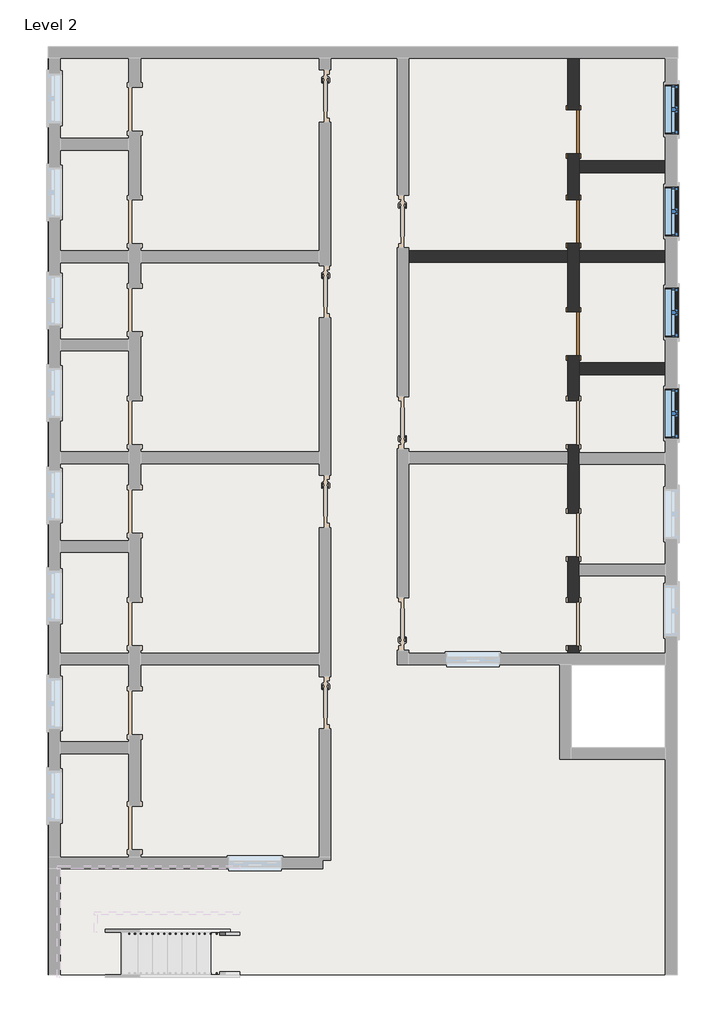
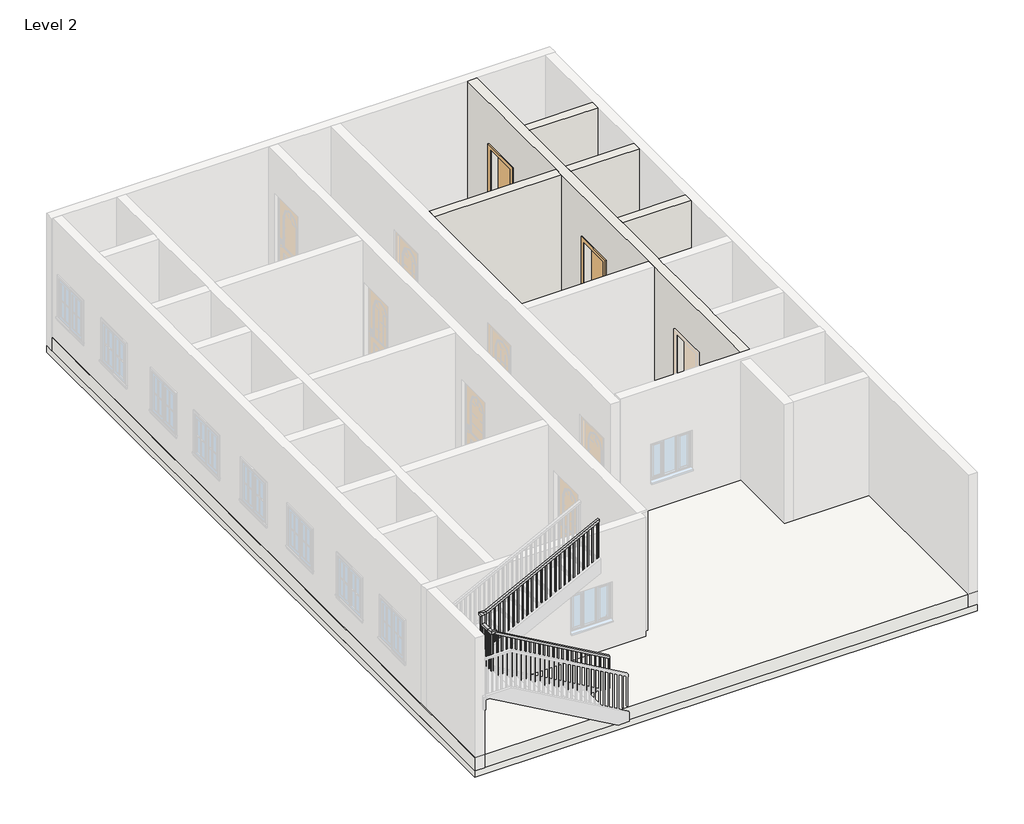
# One storey, part 2 of 4: 5 walls, 4 windows, 3 doors, 1 railing, 1 roof, 1 slab.
"""IFC4 building model written with IfcOpenShell, lengths in millimetres."""

from ifc_helpers import new_model, si_unit, frame, origin, place, context, project, spatial, polyline, outline, extrude, faceted_brep, transform, mapped, element, save
from components import door_53b1b562, window_c29befe5

model = new_model("IFC4")

# Units and contexts
model_context = context("Model", 3, world=origin())
ifc_project = project(units=[si_unit("LENGTHUNIT", "METRE", prefix="MILLI")], contexts=[model_context])

# Site, building, storey
site = spatial("IfcSite", under=ifc_project)
building = spatial("IfcBuilding", under=site)
storey = spatial("IfcBuildingStorey", under=building, Name="Level 2", Elevation=3048.0)

# Doors
placement = place(None, origin())
door_shape = door_53b1b562(model_context)
element("IfcDoor", 1, ObjectType="Single-Flush : 30\" x 80\"", at=placement, inside=storey, context=model_context, shape_type="MappedRepresentation", body=[
    mapped(door_shape, transform((2695.5891134, 6512.9399728, 3048.0), x_axis=(0.0, 1.0, 0.0), y_axis=(-1.0, 0.0, 0.0), z_axis=(0.0, 0.0, 1.0))),
])
element("IfcDoor", 2, ObjectType="Single-Flush : 30\" x 80\"", at=placement, inside=storey, context=model_context, shape_type="MappedRepresentation", body=[
    mapped(door_shape, transform((2695.5891134, 4950.8399728, 3048.0), x_axis=(0.0, 1.0, 0.0), y_axis=(-1.0, 0.0, 0.0), z_axis=(0.0, 0.0, 1.0))),
])
element("IfcDoor", 3, ObjectType="Single-Flush : 30\" x 80\"", at=placement, inside=storey, context=model_context, shape_type="MappedRepresentation", body=[
    mapped(door_shape, transform((2695.5891134, 2995.0399728, 3048.0), x_axis=(0.0, 1.0, 0.0), y_axis=(-1.0, 0.0, 0.0), z_axis=(0.0, 0.0, 1.0))),
])

# Railing
element("IfcRailing", 4, ObjectType="Handrail - Rectangular", at=placement, inside=storey, context=model_context, shape_type="SolidModel", body=[
    faceted_brep([(-3117.2664982, -7482.4600272, 4107.5428571), (-3117.2664982, -7482.4600272, 4049.0339009), (-3117.2664982, -7431.6600272, 4049.0339009), (-3117.2664982, -7431.6600272, 4107.5428571), (-5581.0664982, -7482.4600272, 5515.4285714), (-5631.8664982, -7482.4600272, 5485.9481866), (-5631.8664982, -7431.6600272, 5485.9481866), (-5581.0664982, -7431.6600272, 5515.4285714), (-5581.0664982, -7482.4600272, 5558.9714286), (-5631.8664982, -7482.4600272, 5508.1714286), (-5631.8664982, -7431.6600272, 5508.1714286), (-5581.0664982, -7431.6600272, 5558.9714286), (-5708.0664982, -7482.4600272, 5558.9714286), (-5708.0664982, -7482.4600272, 5508.1714286), (-5657.2664982, -7431.6600272, 5508.1714286), (-5657.2664982, -7431.6600272, 5558.9714286), (-5708.0664982, -7355.4600272, 5558.9714286), (-5708.0664982, -7355.4600272, 5508.1714286), (-5657.2664982, -7355.4600272, 5508.1714286), (-5657.2664982, -7355.4600272, 5558.9714286), (-5708.0664982, -7152.2600272, 5558.9714286), (-5708.0664982, -7101.4600272, 5508.1714286), (-5657.2664982, -7101.4600272, 5508.1714286), (-5657.2664982, -7152.2600272, 5558.9714286), (-5708.0664982, -7152.2600272, 5743.3028571), (-5708.0664982, -7101.4600272, 5692.5028571), (-5657.2664982, -7101.4600272, 5692.5028571), (-5657.2664982, -7152.2600272, 5743.3028571), (-5708.0664982, -7025.2600272, 5743.3028571), (-5708.0664982, -7025.2600272, 5692.5028571), (-5657.2664982, -7076.0600272, 5692.5028571), (-5657.2664982, -7076.0600272, 5743.3028571), (-5581.0664982, -7025.2600272, 5743.3028571), (-5568.769124, -7025.2600272, 5692.5028571), (-5568.769124, -7076.0600272, 5692.5028571), (-5581.0664982, -7076.0600272, 5743.3028571), (-3117.2664982, -7025.2600272, 7010.4), (-3117.2664982, -7076.0600272, 7010.4), (-3117.2664982, -7076.0600272, 6953.2756361), (-3117.2664982, -7025.2600272, 6953.2756361)], [[[0, 1, 2, 3]], [[1, 0, 4, 5]], [[2, 1, 5, 6]], [[3, 2, 6, 7]], [[0, 3, 7, 4]], [[5, 4, 8, 9]], [[6, 5, 9, 10]], [[7, 6, 10, 11]], [[4, 7, 11, 8]], [[9, 8, 12, 13]], [[10, 9, 13, 14]], [[11, 10, 14, 15]], [[8, 11, 15, 12]], [[13, 12, 16, 17]], [[14, 13, 17, 18]], [[15, 14, 18, 19]], [[12, 15, 19, 16]], [[17, 16, 20, 21]], [[18, 17, 21, 22]], [[19, 18, 22, 23]], [[16, 19, 23, 20]], [[21, 20, 24, 25]], [[22, 21, 25, 26]], [[23, 22, 26, 27]], [[20, 23, 27, 24]], [[25, 24, 28, 29]], [[26, 25, 29, 30]], [[27, 26, 30, 31]], [[24, 27, 31, 28]], [[29, 28, 32, 33]], [[30, 29, 33, 34]], [[31, 30, 34, 35]], [[28, 31, 35, 32]], [[36, 37, 38, 39]], [[33, 32, 36, 39]], [[34, 33, 39, 38]], [[35, 34, 38, 37]], [[32, 35, 37, 36]]]),
    extrude(outline(polyline([(6945.1113504, -3133.1414982), (6935.3142076, -3152.1914982), (5950.8571429, -3152.1914982), (5950.8571429, -3133.1414982), (6945.1113504, -3133.1414982)])), frame((0.0, -7060.1850272, 0.0), z_axis=(0.0, 1.0, 0.0), x_axis=(0.0, 0.0, 1.0)), (0.0, 0.0, 1.0), 19.05),
    extrude(outline(polyline([(6892.8599218, -3234.7414982), (6883.062779, -3253.7914982), (5950.8571429, -3253.7914982), (5950.8571429, -3234.7414982), (6892.8599218, -3234.7414982)])), frame((0.0, -7060.1850272, 0.0), z_axis=(0.0, 1.0, 0.0), x_axis=(0.0, 0.0, 1.0)), (0.0, 0.0, 1.0), 19.05),
    extrude(outline(polyline([(6840.6084933, -3336.3414982), (6830.8113504, -3355.3914982), (5950.8571429, -3355.3914982), (5950.8571429, -3336.3414982), (6840.6084933, -3336.3414982)])), frame((0.0, -7060.1850272, 0.0), z_axis=(0.0, 1.0, 0.0), x_axis=(0.0, 0.0, 1.0)), (0.0, 0.0, 1.0), 19.05),
    extrude(outline(polyline([(6788.3570647, -3437.9414982), (6778.5599218, -3456.9914982), (5805.7142857, -3456.9914982), (5805.7142857, -3437.9414982), (6788.3570647, -3437.9414982)])), frame((0.0, -7060.1850272, 0.0), z_axis=(0.0, 1.0, 0.0), x_axis=(0.0, 0.0, 1.0)), (0.0, 0.0, 1.0), 19.05),
    extrude(outline(polyline([(6736.1056361, -3539.5414982), (6726.3084933, -3558.5914982), (5805.7142857, -3558.5914982), (5805.7142857, -3539.5414982), (6736.1056361, -3539.5414982)])), frame((0.0, -7060.1850272, 0.0), z_axis=(0.0, 1.0, 0.0), x_axis=(0.0, 0.0, 1.0)), (0.0, 0.0, 1.0), 19.05),
    extrude(outline(polyline([(6683.8542076, -3641.1414982), (6674.0570647, -3660.1914982), (5660.5714286, -3660.1914982), (5660.5714286, -3641.1414982), (6683.8542076, -3641.1414982)])), frame((0.0, -7060.1850272, 0.0), z_axis=(0.0, 1.0, 0.0), x_axis=(0.0, 0.0, 1.0)), (0.0, 0.0, 1.0), 19.05),
    extrude(outline(polyline([(6631.602779, -3742.7414982), (6621.8056361, -3761.7914982), (5660.5714286, -3761.7914982), (5660.5714286, -3742.7414982), (6631.602779, -3742.7414982)])), frame((0.0, -7060.1850272, 0.0), z_axis=(0.0, 1.0, 0.0), x_axis=(0.0, 0.0, 1.0)), (0.0, 0.0, 1.0), 19.05),
    extrude(outline(polyline([(6579.3513504, -3844.3414982), (6569.5542076, -3863.3914982), (5660.5714286, -3863.3914982), (5660.5714286, -3844.3414982), (6579.3513504, -3844.3414982)])), frame((0.0, -7060.1850272, 0.0), z_axis=(0.0, 1.0, 0.0), x_axis=(0.0, 0.0, 1.0)), (0.0, 0.0, 1.0), 19.05),
    extrude(outline(polyline([(6527.0999218, -3945.9414982), (6517.302779, -3964.9914982), (5660.5714286, -3964.9914982), (5660.5714286, -3945.9414982), (6527.0999218, -3945.9414982)])), frame((0.0, -7060.1850272, 0.0), z_axis=(0.0, 1.0, 0.0), x_axis=(0.0, 0.0, 1.0)), (0.0, 0.0, 1.0), 19.05),
    extrude(outline(polyline([(6474.8484933, -4047.5414982), (6465.0513504, -4066.5914982), (5660.5714286, -4066.5914982), (5660.5714286, -4047.5414982), (6474.8484933, -4047.5414982)])), frame((0.0, -7060.1850272, 0.0), z_axis=(0.0, 1.0, 0.0), x_axis=(0.0, 0.0, 1.0)), (0.0, 0.0, 1.0), 19.05),
    extrude(outline(polyline([(6422.5970647, -4149.1414982), (6412.7999218, -4168.1914982), (5515.4285714, -4168.1914982), (5515.4285714, -4149.1414982), (6422.5970647, -4149.1414982)])), frame((0.0, -7060.1850272, 0.0), z_axis=(0.0, 1.0, 0.0), x_axis=(0.0, 0.0, 1.0)), (0.0, 0.0, 1.0), 19.05),
    extrude(outline(polyline([(6370.3456361, -4250.7414982), (6360.5484933, -4269.7914982), (5515.4285714, -4269.7914982), (5515.4285714, -4250.7414982), (6370.3456361, -4250.7414982)])), frame((0.0, -7060.1850272, 0.0), z_axis=(0.0, 1.0, 0.0), x_axis=(0.0, 0.0, 1.0)), (0.0, 0.0, 1.0), 19.05),
    extrude(outline(polyline([(6318.0942076, -4352.3414982), (6308.2970647, -4371.3914982), (5515.4285714, -4371.3914982), (5515.4285714, -4352.3414982), (6318.0942076, -4352.3414982)])), frame((0.0, -7060.1850272, 0.0), z_axis=(0.0, 1.0, 0.0), x_axis=(0.0, 0.0, 1.0)), (0.0, 0.0, 1.0), 19.05),
    extrude(outline(polyline([(6265.842779, -4453.9414982), (6256.0456361, -4472.9914982), (5370.2857143, -4472.9914982), (5370.2857143, -4453.9414982), (6265.842779, -4453.9414982)])), frame((0.0, -7060.1850272, 0.0), z_axis=(0.0, 1.0, 0.0), x_axis=(0.0, 0.0, 1.0)), (0.0, 0.0, 1.0), 19.05),
    extrude(outline(polyline([(6213.5913504, -4555.5414982), (6203.7942076, -4574.5914982), (5370.2857143, -4574.5914982), (5370.2857143, -4555.5414982), (6213.5913504, -4555.5414982)])), frame((0.0, -7060.1850272, 0.0), z_axis=(0.0, 1.0, 0.0), x_axis=(0.0, 0.0, 1.0)), (0.0, 0.0, 1.0), 19.05),
    extrude(outline(polyline([(6161.3399218, -4657.1414982), (6151.542779, -4676.1914982), (5225.1428571, -4676.1914982), (5225.1428571, -4657.1414982), (6161.3399218, -4657.1414982)])), frame((0.0, -7060.1850272, 0.0), z_axis=(0.0, 1.0, 0.0), x_axis=(0.0, 0.0, 1.0)), (0.0, 0.0, 1.0), 19.05),
    extrude(outline(polyline([(6109.0884933, -4758.7414982), (6099.2913504, -4777.7914982), (5225.1428571, -4777.7914982), (5225.1428571, -4758.7414982), (6109.0884933, -4758.7414982)])), frame((0.0, -7060.1850272, 0.0), z_axis=(0.0, 1.0, 0.0), x_axis=(0.0, 0.0, 1.0)), (0.0, 0.0, 1.0), 19.05),
    extrude(outline(polyline([(6056.8370647, -4860.3414982), (6047.0399218, -4879.3914982), (5225.1428571, -4879.3914982), (5225.1428571, -4860.3414982), (6056.8370647, -4860.3414982)])), frame((0.0, -7060.1850272, 0.0), z_axis=(0.0, 1.0, 0.0), x_axis=(0.0, 0.0, 1.0)), (0.0, 0.0, 1.0), 19.05),
    extrude(outline(polyline([(6004.5856361, -4961.9414982), (5994.7884933, -4980.9914982), (5080.0, -4980.9914982), (5080.0, -4961.9414982), (6004.5856361, -4961.9414982)])), frame((0.0, -7060.1850272, 0.0), z_axis=(0.0, 1.0, 0.0), x_axis=(0.0, 0.0, 1.0)), (0.0, 0.0, 1.0), 19.05),
    extrude(outline(polyline([(5952.3342076, -5063.5414982), (5942.5370647, -5082.5914982), (5080.0, -5082.5914982), (5080.0, -5063.5414982), (5952.3342076, -5063.5414982)])), frame((0.0, -7060.1850272, 0.0), z_axis=(0.0, 1.0, 0.0), x_axis=(0.0, 0.0, 1.0)), (0.0, 0.0, 1.0), 19.05),
    extrude(outline(polyline([(5900.082779, -5165.1414982), (5890.2856361, -5184.1914982), (4934.8571429, -5184.1914982), (4934.8571429, -5165.1414982), (5900.082779, -5165.1414982)])), frame((0.0, -7060.1850272, 0.0), z_axis=(0.0, 1.0, 0.0), x_axis=(0.0, 0.0, 1.0)), (0.0, 0.0, 1.0), 19.05),
    extrude(outline(polyline([(5847.8313504, -5266.7414982), (5838.0342076, -5285.7914982), (4934.8571429, -5285.7914982), (4934.8571429, -5266.7414982), (5847.8313504, -5266.7414982)])), frame((0.0, -7060.1850272, 0.0), z_axis=(0.0, 1.0, 0.0), x_axis=(0.0, 0.0, 1.0)), (0.0, 0.0, 1.0), 19.05),
    extrude(outline(polyline([(5795.5799218, -5368.3414982), (5785.782779, -5387.3914982), (4934.8571429, -5387.3914982), (4934.8571429, -5368.3414982), (5795.5799218, -5368.3414982)])), frame((0.0, -7060.1850272, 0.0), z_axis=(0.0, 1.0, 0.0), x_axis=(0.0, 0.0, 1.0)), (0.0, 0.0, 1.0), 19.05),
    extrude(outline(polyline([(5743.3284933, -5469.9414982), (5733.5313504, -5488.9914982), (4789.7142857, -5488.9914982), (4789.7142857, -5469.9414982), (5743.3284933, -5469.9414982)])), frame((0.0, -7060.1850272, 0.0), z_axis=(0.0, 1.0, 0.0), x_axis=(0.0, 0.0, 1.0)), (0.0, 0.0, 1.0), 19.05),
    extrude(outline(polyline([(5691.0770647, -5571.5414982), (5681.2799218, -5590.5914982), (4789.7142857, -5590.5914982), (4789.7142857, -5571.5414982), (5691.0770647, -5571.5414982)])), frame((0.0, -7060.1850272, 0.0), z_axis=(0.0, 1.0, 0.0), x_axis=(0.0, 0.0, 1.0)), (0.0, 0.0, 1.0), 19.05),
    extrude(outline(polyline([(-5673.1414982, -7161.7850272), (-5692.1914982, -7161.7850272), (-5692.1914982, -7142.7350272), (-5673.1414982, -7142.7350272), (-5673.1414982, -7161.7850272)])), frame((0.0, 0.0, 4644.5714286), z_axis=(0.0, 0.0, 1.0), x_axis=(1.0, 0.0, 0.0)), (0.0, 0.0, 1.0), 863.6),
    extrude(outline(polyline([(-5673.1414982, -7263.3850272), (-5692.1914982, -7263.3850272), (-5692.1914982, -7244.3350272), (-5673.1414982, -7244.3350272), (-5673.1414982, -7263.3850272)])), frame((0.0, 0.0, 4644.5714286), z_axis=(0.0, 0.0, 1.0), x_axis=(1.0, 0.0, 0.0)), (0.0, 0.0, 1.0), 863.6),
    extrude(outline(polyline([(-5673.1414982, -7364.9850272), (-5692.1914982, -7364.9850272), (-5692.1914982, -7345.9350272), (-5673.1414982, -7345.9350272), (-5673.1414982, -7364.9850272)])), frame((0.0, 0.0, 4644.5714286), z_axis=(0.0, 0.0, 1.0), x_axis=(1.0, 0.0, 0.0)), (0.0, 0.0, 1.0), 863.6),
    extrude(outline(polyline([(-5647.7414982, -7447.5350272), (-5647.7414982, -7466.5850272), (-5666.7914982, -7466.5850272), (-5666.7914982, -7447.5350272), (-5647.7414982, -7447.5350272)])), frame((0.0, 0.0, 4644.5714286), z_axis=(0.0, 0.0, 1.0), x_axis=(1.0, 0.0, 0.0)), (0.0, 0.0, 1.0), 863.6),
    extrude(outline(polyline([(5436.9624723, -5546.1414982), (5447.8481866, -5565.1914982), (4499.4285714, -5565.1914982), (4499.4285714, -5546.1414982), (5436.9624723, -5546.1414982)])), frame((0.0, -7466.5850272, 0.0), z_axis=(0.0, 1.0, 0.0), x_axis=(0.0, 0.0, 1.0)), (0.0, 0.0, 1.0), 19.05),
    extrude(outline(polyline([(5378.9053295, -5444.5414982), (5389.7910438, -5463.5914982), (4499.4285714, -5463.5914982), (4499.4285714, -5444.5414982), (5378.9053295, -5444.5414982)])), frame((0.0, -7466.5850272, 0.0), z_axis=(0.0, 1.0, 0.0), x_axis=(0.0, 0.0, 1.0)), (0.0, 0.0, 1.0), 19.05),
    extrude(outline(polyline([(5320.8481866, -5342.9414982), (5331.7339009, -5361.9914982), (4354.2857143, -5361.9914982), (4354.2857143, -5342.9414982), (5320.8481866, -5342.9414982)])), frame((0.0, -7466.5850272, 0.0), z_axis=(0.0, 1.0, 0.0), x_axis=(0.0, 0.0, 1.0)), (0.0, 0.0, 1.0), 19.05),
    extrude(outline(polyline([(5262.7910438, -5241.3414982), (5273.6767581, -5260.3914982), (4354.2857143, -5260.3914982), (4354.2857143, -5241.3414982), (5262.7910438, -5241.3414982)])), frame((0.0, -7466.5850272, 0.0), z_axis=(0.0, 1.0, 0.0), x_axis=(0.0, 0.0, 1.0)), (0.0, 0.0, 1.0), 19.05),
    extrude(outline(polyline([(5204.7339009, -5139.7414982), (5215.6196152, -5158.7914982), (4354.2857143, -5158.7914982), (4354.2857143, -5139.7414982), (5204.7339009, -5139.7414982)])), frame((0.0, -7466.5850272, 0.0), z_axis=(0.0, 1.0, 0.0), x_axis=(0.0, 0.0, 1.0)), (0.0, 0.0, 1.0), 19.05),
    extrude(outline(polyline([(5146.6767581, -5038.1414982), (5157.5624723, -5057.1914982), (4209.1428571, -5057.1914982), (4209.1428571, -5038.1414982), (5146.6767581, -5038.1414982)])), frame((0.0, -7466.5850272, 0.0), z_axis=(0.0, 1.0, 0.0), x_axis=(0.0, 0.0, 1.0)), (0.0, 0.0, 1.0), 19.05),
    extrude(outline(polyline([(5088.6196152, -4936.5414982), (5099.5053295, -4955.5914982), (4209.1428571, -4955.5914982), (4209.1428571, -4936.5414982), (5088.6196152, -4936.5414982)])), frame((0.0, -7466.5850272, 0.0), z_axis=(0.0, 1.0, 0.0), x_axis=(0.0, 0.0, 1.0)), (0.0, 0.0, 1.0), 19.05),
    extrude(outline(polyline([(5030.5624723, -4834.9414982), (5041.4481866, -4853.9914982), (4064.0, -4853.9914982), (4064.0, -4834.9414982), (5030.5624723, -4834.9414982)])), frame((0.0, -7466.5850272, 0.0), z_axis=(0.0, 1.0, 0.0), x_axis=(0.0, 0.0, 1.0)), (0.0, 0.0, 1.0), 19.05),
    extrude(outline(polyline([(4972.5053295, -4733.3414982), (4983.3910438, -4752.3914982), (4064.0, -4752.3914982), (4064.0, -4733.3414982), (4972.5053295, -4733.3414982)])), frame((0.0, -7466.5850272, 0.0), z_axis=(0.0, 1.0, 0.0), x_axis=(0.0, 0.0, 1.0)), (0.0, 0.0, 1.0), 19.05),
    extrude(outline(polyline([(4914.4481866, -4631.7414982), (4925.3339009, -4650.7914982), (4064.0, -4650.7914982), (4064.0, -4631.7414982), (4914.4481866, -4631.7414982)])), frame((0.0, -7466.5850272, 0.0), z_axis=(0.0, 1.0, 0.0), x_axis=(0.0, 0.0, 1.0)), (0.0, 0.0, 1.0), 19.05),
    extrude(outline(polyline([(4856.3910438, -4530.1414982), (4867.2767581, -4549.1914982), (3918.8571429, -4549.1914982), (3918.8571429, -4530.1414982), (4856.3910438, -4530.1414982)])), frame((0.0, -7466.5850272, 0.0), z_axis=(0.0, 1.0, 0.0), x_axis=(0.0, 0.0, 1.0)), (0.0, 0.0, 1.0), 19.05),
    extrude(outline(polyline([(4798.3339009, -4428.5414982), (4809.2196152, -4447.5914982), (3918.8571429, -4447.5914982), (3918.8571429, -4428.5414982), (4798.3339009, -4428.5414982)])), frame((0.0, -7466.5850272, 0.0), z_axis=(0.0, 1.0, 0.0), x_axis=(0.0, 0.0, 1.0)), (0.0, 0.0, 1.0), 19.05),
    extrude(outline(polyline([(4740.2767581, -4326.9414982), (4751.1624723, -4345.9914982), (3773.7142857, -4345.9914982), (3773.7142857, -4326.9414982), (4740.2767581, -4326.9414982)])), frame((0.0, -7466.5850272, 0.0), z_axis=(0.0, 1.0, 0.0), x_axis=(0.0, 0.0, 1.0)), (0.0, 0.0, 1.0), 19.05),
    extrude(outline(polyline([(4682.2196152, -4225.3414982), (4693.1053295, -4244.3914982), (3773.7142857, -4244.3914982), (3773.7142857, -4225.3414982), (4682.2196152, -4225.3414982)])), frame((0.0, -7466.5850272, 0.0), z_axis=(0.0, 1.0, 0.0), x_axis=(0.0, 0.0, 1.0)), (0.0, 0.0, 1.0), 19.05),
    extrude(outline(polyline([(4624.1624723, -4123.7414982), (4635.0481866, -4142.7914982), (3773.7142857, -4142.7914982), (3773.7142857, -4123.7414982), (4624.1624723, -4123.7414982)])), frame((0.0, -7466.5850272, 0.0), z_axis=(0.0, 1.0, 0.0), x_axis=(0.0, 0.0, 1.0)), (0.0, 0.0, 1.0), 19.05),
    extrude(outline(polyline([(4566.1053295, -4022.1414982), (4576.9910438, -4041.1914982), (3628.5714286, -4041.1914982), (3628.5714286, -4022.1414982), (4566.1053295, -4022.1414982)])), frame((0.0, -7466.5850272, 0.0), z_axis=(0.0, 1.0, 0.0), x_axis=(0.0, 0.0, 1.0)), (0.0, 0.0, 1.0), 19.05),
    extrude(outline(polyline([(4508.0481866, -3920.5414982), (4518.9339009, -3939.5914982), (3628.5714286, -3939.5914982), (3628.5714286, -3920.5414982), (4508.0481866, -3920.5414982)])), frame((0.0, -7466.5850272, 0.0), z_axis=(0.0, 1.0, 0.0), x_axis=(0.0, 0.0, 1.0)), (0.0, 0.0, 1.0), 19.05),
    extrude(outline(polyline([(4449.9910438, -3818.9414982), (4460.8767581, -3837.9914982), (3483.4285714, -3837.9914982), (3483.4285714, -3818.9414982), (4449.9910438, -3818.9414982)])), frame((0.0, -7466.5850272, 0.0), z_axis=(0.0, 1.0, 0.0), x_axis=(0.0, 0.0, 1.0)), (0.0, 0.0, 1.0), 19.05),
    extrude(outline(polyline([(4391.9339009, -3717.3414982), (4402.8196152, -3736.3914982), (3483.4285714, -3736.3914982), (3483.4285714, -3717.3414982), (4391.9339009, -3717.3414982)])), frame((0.0, -7466.5850272, 0.0), z_axis=(0.0, 1.0, 0.0), x_axis=(0.0, 0.0, 1.0)), (0.0, 0.0, 1.0), 19.05),
    extrude(outline(polyline([(4333.8767581, -3615.7414982), (4344.7624723, -3634.7914982), (3483.4285714, -3634.7914982), (3483.4285714, -3615.7414982), (4333.8767581, -3615.7414982)])), frame((0.0, -7466.5850272, 0.0), z_axis=(0.0, 1.0, 0.0), x_axis=(0.0, 0.0, 1.0)), (0.0, 0.0, 1.0), 19.05),
    extrude(outline(polyline([(4275.8196152, -3514.1414982), (4286.7053295, -3533.1914982), (3338.2857143, -3533.1914982), (3338.2857143, -3514.1414982), (4275.8196152, -3514.1414982)])), frame((0.0, -7466.5850272, 0.0), z_axis=(0.0, 1.0, 0.0), x_axis=(0.0, 0.0, 1.0)), (0.0, 0.0, 1.0), 19.05),
    extrude(outline(polyline([(4217.7624723, -3412.5414982), (4228.6481866, -3431.5914982), (3338.2857143, -3431.5914982), (3338.2857143, -3412.5414982), (4217.7624723, -3412.5414982)])), frame((0.0, -7466.5850272, 0.0), z_axis=(0.0, 1.0, 0.0), x_axis=(0.0, 0.0, 1.0)), (0.0, 0.0, 1.0), 19.05),
    extrude(outline(polyline([(4159.7053295, -3310.9414982), (4170.5910438, -3329.9914982), (3193.1428571, -3329.9914982), (3193.1428571, -3310.9414982), (4159.7053295, -3310.9414982)])), frame((0.0, -7466.5850272, 0.0), z_axis=(0.0, 1.0, 0.0), x_axis=(0.0, 0.0, 1.0)), (0.0, 0.0, 1.0), 19.05),
    extrude(outline(polyline([(4101.6481866, -3209.3414982), (4112.5339009, -3228.3914982), (3193.1428571, -3228.3914982), (3193.1428571, -3209.3414982), (4101.6481866, -3209.3414982)])), frame((0.0, -7466.5850272, 0.0), z_axis=(0.0, 1.0, 0.0), x_axis=(0.0, 0.0, 1.0)), (0.0, 0.0, 1.0), 19.05),
    extrude(outline(polyline([(-5673.1414982, -7060.1850272), (-5692.1914982, -7060.1850272), (-5692.1914982, -7041.1350272), (-5673.1414982, -7041.1350272), (-5673.1414982, -7060.1850272)])), frame((0.0, 0.0, 4644.5714286), z_axis=(0.0, 0.0, 1.0), x_axis=(1.0, 0.0, 0.0)), (0.0, 0.0, 1.0), 1047.9314286),
    extrude(outline(polyline([(-5673.1414982, -7447.5350272), (-5673.1414982, -7466.5850272), (-5692.1914982, -7466.5850272), (-5692.1914982, -7447.5350272), (-5673.1414982, -7447.5350272)])), frame((0.0, 0.0, 4644.5714286), z_axis=(0.0, 0.0, 1.0), x_axis=(1.0, 0.0, 0.0)), (0.0, 0.0, 1.0), 863.6),
    extrude(outline(polyline([(6953.2756361, -3117.2664982), (6943.4784933, -3136.3164982), (5950.8571429, -3136.3164982), (5950.8571429, -3117.2664982), (6953.2756361, -3117.2664982)])), frame((0.0, -7060.1850272, 0.0), z_axis=(0.0, 1.0, 0.0), x_axis=(0.0, 0.0, 1.0)), (0.0, 0.0, 1.0), 19.05),
    extrude(outline(polyline([(4049.0339009, -3117.2664982), (4059.9196152, -3136.3164982), (3193.1428571, -3136.3164982), (3193.1428571, -3117.2664982), (4049.0339009, -3117.2664982)])), frame((0.0, -7466.5850272, 0.0), z_axis=(0.0, 1.0, 0.0), x_axis=(0.0, 0.0, 1.0)), (0.0, 0.0, 1.0), 19.05),
])

# Roof
element("IfcRoof", 5, ObjectType="Generic - 12\"", at=placement, inside=storey, context=model_context, shape_type="SweptSolid", body=[
    extrude(outline(polyline([(-6461.1108866, -8168.2600272), (-6461.1108866, 7998.8399728), (4498.9891134, 7998.8399728), (4498.9891134, -8168.2600272), (-6461.1108866, -8168.2600272)]), holes=[polyline([(4295.7891134, -2770.7600272), (2657.4891134, -2770.7600272), (2657.4891134, -4218.5600272), (4295.7891134, -4218.5600272), (4295.7891134, -2770.7600272)])]), frame((0.0, 0.0, 3048.0), z_axis=(0.0, 0.0, 1.0), x_axis=(1.0, 0.0, 0.0)), (0.0, 0.0, 1.0), 304.8),
])

# Slab
element("IfcSlab", 6, ObjectType="Generic - 12\"", at=placement, inside=storey, context=model_context, shape_type="SweptSolid", body=[
    extrude(outline(polyline([(4498.9891134, 7998.8399728), (4498.9891134, -8168.2600272), (-6461.1108866, -8168.2600272), (-6461.1108866, 7998.8399728), (4498.9891134, 7998.8399728)]), holes=[polyline([(4295.7891134, -2770.7600272), (2657.4891134, -2770.7600272), (2657.4891134, -4218.5600272), (4295.7891134, -4218.5600272), (4295.7891134, -2770.7600272)])]), frame((0.0, 0.0, 2895.6), z_axis=(0.0, 0.0, 1.0), x_axis=(1.0, 0.0, 0.0)), (0.0, 0.0, 1.0), 152.4),
])

# Walls
element("IfcWall", 7, ObjectType="4.5\" p", at=placement, inside=storey, context=model_context, shape_type="Brep", body=[
    faceted_brep([(2593.9891134, -2440.5600272, 5080.0), (2593.9891134, -2440.5600272, 3048.0), (2593.9891134, -2567.5600272, 3048.0), (2593.9891134, -2567.5600272, 6096.0), (2593.9891134, 734.4399728, 6096.0), (2593.9891134, 937.6399728, 6096.0), (2593.9891134, 4239.6399728, 6096.0), (2593.9891134, 4442.8399728, 6096.0), (2593.9891134, 7795.6399728, 6096.0), (2593.9891134, 7795.6399728, 3048.0), (2593.9891134, 6893.9399728, 3048.0), (2593.9891134, 6893.9399728, 5080.0), (2593.9891134, 6131.9399728, 5080.0), (2593.9891134, 6131.9399728, 3048.0), (2593.9891134, 5331.8399728, 3048.0), (2593.9891134, 5331.8399728, 5080.0), (2593.9891134, 4569.8399728, 5080.0), (2593.9891134, 4569.8399728, 3048.0), (2593.9891134, 4442.8399728, 3048.0), (2593.9891134, 4239.6399728, 3048.0), (2593.9891134, 3376.0399728, 3048.0), (2593.9891134, 3376.0399728, 5080.0), (2593.9891134, 2614.0399728, 5080.0), (2593.9891134, 2614.0399728, 3048.0), (2593.9891134, 1826.6399728, 3048.0), (2593.9891134, 1826.6399728, 5080.0), (2593.9891134, 1064.6399728, 5080.0), (2593.9891134, 1064.6399728, 3048.0), (2593.9891134, 937.6399728, 3048.0), (2593.9891134, 734.4399728, 3048.0), (2593.9891134, -129.1600272, 3048.0), (2593.9891134, -129.1600272, 5080.0), (2593.9891134, -891.1600272, 5080.0), (2593.9891134, -891.1600272, 3048.0), (2593.9891134, -1678.5600272, 3048.0), (2593.9891134, -1678.5600272, 5080.0), (2797.1891134, -2567.5600272, 3048.0), (2797.1891134, -2440.5600272, 3048.0), (2797.1891134, -2440.5600272, 5080.0), (2797.1891134, -1678.5600272, 5080.0), (2797.1891134, -1678.5600272, 3048.0), (2797.1891134, -1221.3600272, 3048.0), (2797.1891134, -1018.1600272, 3048.0), (2797.1891134, -891.1600272, 3048.0), (2797.1891134, -891.1600272, 5080.0), (2797.1891134, -129.1600272, 5080.0), (2797.1891134, -129.1600272, 3048.0), (2797.1891134, 721.7399728, 3048.0), (2797.1891134, 924.9399728, 3048.0), (2797.1891134, 1064.6399728, 3048.0), (2797.1891134, 1064.6399728, 5080.0), (2797.1891134, 1826.6399728, 5080.0), (2797.1891134, 1826.6399728, 3048.0), (2797.1891134, 2283.8399728, 3048.0), (2797.1891134, 2487.0399728, 3048.0), (2797.1891134, 2614.0399728, 3048.0), (2797.1891134, 2614.0399728, 5080.0), (2797.1891134, 3376.0399728, 5080.0), (2797.1891134, 3376.0399728, 3048.0), (2797.1891134, 4239.6399728, 3048.0), (2797.1891134, 4442.8399728, 3048.0), (2797.1891134, 4569.8399728, 3048.0), (2797.1891134, 4569.8399728, 5080.0), (2797.1891134, 5331.8399728, 5080.0), (2797.1891134, 5331.8399728, 3048.0), (2797.1891134, 5801.7399728, 3048.0), (2797.1891134, 6004.9399728, 3048.0), (2797.1891134, 6131.9399728, 3048.0), (2797.1891134, 6131.9399728, 5080.0), (2797.1891134, 6893.9399728, 5080.0), (2797.1891134, 6893.9399728, 3048.0), (2797.1891134, 7795.6399728, 3048.0), (2797.1891134, 7795.6399728, 6096.0), (2797.1891134, 6004.9399728, 6096.0), (2797.1891134, 5801.7399728, 6096.0), (2797.1891134, 4442.8399728, 6096.0), (2797.1891134, 4239.6399728, 6096.0), (2797.1891134, 2487.0399728, 6096.0), (2797.1891134, 2283.8399728, 6096.0), (2797.1891134, 924.9399728, 6096.0), (2797.1891134, 721.7399728, 6096.0), (2797.1891134, -1018.1600272, 6096.0), (2797.1891134, -1221.3600272, 6096.0), (2797.1891134, -2567.5600272, 6096.0)], [[[0, 1, 2, 3, 4, 5, 6, 7, 8, 9, 10, 11, 12, 13, 14, 15, 16, 17, 18, 19, 20, 21, 22, 23, 24, 25, 26, 27, 28, 29, 30, 31, 32, 33, 34, 35]], [[36, 37, 38, 39, 40, 41, 42, 43, 44, 45, 46, 47, 48, 49, 50, 51, 52, 53, 54, 55, 56, 57, 58, 59, 60, 61, 62, 63, 64, 65, 66, 67, 68, 69, 70, 71, 72, 73, 74, 75, 76, 77, 78, 79, 80, 81, 82, 83]], [[71, 70, 10, 9]], [[67, 66, 65, 64, 14, 13]], [[61, 60, 59, 58, 20, 19, 18, 17]], [[55, 54, 53, 52, 24, 23]], [[30, 29, 28, 27, 49, 48, 47, 46]], [[34, 33, 43, 42, 41, 40]], [[2, 1, 37, 36]], [[8, 7, 6, 5, 4, 3, 83, 82, 81, 80, 79, 78, 77, 76, 75, 74, 73, 72]], [[9, 8, 72, 71]], [[3, 2, 36, 83]], [[11, 10, 70, 69]], [[12, 11, 69, 68]], [[13, 12, 68, 67]], [[15, 14, 64, 63]], [[16, 15, 63, 62]], [[17, 16, 62, 61]], [[21, 20, 58, 57]], [[22, 21, 57, 56]], [[23, 22, 56, 55]], [[25, 24, 52, 51]], [[26, 25, 51, 50]], [[27, 26, 50, 49]], [[44, 43, 33, 32]], [[45, 44, 32, 31]], [[46, 45, 31, 30]], [[38, 37, 1, 0]], [[39, 38, 0, 35]], [[40, 39, 35, 34]]]),
])
element("IfcWall", 8, ObjectType="4.5\" p", at=placement, inside=storey, context=model_context, shape_type="SweptSolid", body=[
    extrude(outline(polyline([(4295.7891134, 5801.7399728), (2797.1891134, 5801.7399728), (2797.1891134, 6004.9399728), (4295.7891134, 6004.9399728), (4295.7891134, 5801.7399728)])), frame((0.0, 0.0, 3048.0), z_axis=(0.0, 0.0, 1.0), x_axis=(1.0, 0.0, 0.0)), (0.0, 0.0, 1.0), 3048.0),
])
element("IfcWall", 9, ObjectType="4.5\" p", at=placement, inside=storey, context=model_context, shape_type="SweptSolid", body=[
    extrude(outline(polyline([(4295.7891134, 4239.6399728), (2797.1891134, 4239.6399728), (2797.1891134, 4442.8399728), (4295.7891134, 4442.8399728), (4295.7891134, 4239.6399728)])), frame((0.0, 0.0, 3048.0), z_axis=(0.0, 0.0, 1.0), x_axis=(1.0, 0.0, 0.0)), (0.0, 0.0, 1.0), 3048.0),
])
element("IfcWall", 10, ObjectType="4.5\" p", at=placement, inside=storey, context=model_context, shape_type="SweptSolid", body=[
    extrude(outline(polyline([(4295.7891134, 2283.8399728), (2797.1891134, 2283.8399728), (2797.1891134, 2487.0399728), (4295.7891134, 2487.0399728), (4295.7891134, 2283.8399728)])), frame((0.0, 0.0, 3048.0), z_axis=(0.0, 0.0, 1.0), x_axis=(1.0, 0.0, 0.0)), (0.0, 0.0, 1.0), 3048.0),
])
element("IfcWall", 11, ObjectType="4.5\" p", at=placement, inside=storey, context=model_context, shape_type="SweptSolid", body=[
    extrude(outline(polyline([(2593.9891134, 4239.6399728), (-174.6108866, 4239.6399728), (-174.6108866, 4442.8399728), (2593.9891134, 4442.8399728), (2593.9891134, 4239.6399728)])), frame((0.0, 0.0, 3048.0), z_axis=(0.0, 0.0, 1.0), x_axis=(1.0, 0.0, 0.0)), (0.0, 0.0, 1.0), 3048.0),
])

# Windows
window_shape = window_c29befe5(model_context)
element("IfcWindow", 12, ObjectType="Window-Casement-Double : 34\" x 36\"", at=placement, inside=storey, context=model_context, shape_type="MappedRepresentation", body=[
    mapped(window_shape, transform((4397.3891134, 1604.3899728, 3048.0), x_axis=(0.0, -1.0, 0.0), y_axis=(1.0, 0.0, 0.0), z_axis=(0.0, 0.0, 1.0))),
])
element("IfcWindow", 13, ObjectType="Window-Casement-Double : 34\" x 36\"", at=placement, inside=storey, context=model_context, shape_type="MappedRepresentation", body=[
    mapped(window_shape, transform((4397.3891134, 3363.3399728, 3048.0), x_axis=(0.0, -1.0, 0.0), y_axis=(1.0, 0.0, 0.0), z_axis=(0.0, 0.0, 1.0))),
])
element("IfcWindow", 14, ObjectType="Window-Casement-Double : 34\" x 36\"", at=placement, inside=storey, context=model_context, shape_type="MappedRepresentation", body=[
    mapped(window_shape, transform((4397.3891134, 5122.2899728, 3048.0), x_axis=(0.0, -1.0, 0.0), y_axis=(1.0, 0.0, 0.0), z_axis=(0.0, 0.0, 1.0))),
])
element("IfcWindow", 15, ObjectType="Window-Casement-Double : 34\" x 36\"", at=placement, inside=storey, context=model_context, shape_type="MappedRepresentation", body=[
    mapped(window_shape, transform((4397.3891134, 6900.2899728, 3048.0), x_axis=(0.0, -1.0, 0.0), y_axis=(1.0, 0.0, 0.0), z_axis=(0.0, 0.0, 1.0))),
])

save(model, "model.ifc")

# Revit data of these elements
# Type "Single-Flush : 30\" x 80\""
#   Type Mark = "5"
#   Construction Type Id = "MDOOR"
#   Assembly Code = "C1020"
#   Analytic Construction = "Metal"
#   Thickness = 0' - 2"
#   Heat Transfer Coefficient (U) = 0.651978 BTU/(h·ft²·°F)
#   Height = 6' - 8"
#   Trim Projection Ext = 0' - 1"
#   Trim Projection Int = 0' - 1"
#   Trim Width = 0' - 3"
#   Width = 2' - 6"
#   Define Thermal Properties by = 1
#   Define Thermal Properties by = 1
#   Door Material = Door - Panel
#   Frame Material = Door - Frame
#   Visual Light Transmittance = 0
#   Solar Heat Gain Coefficient = 0
#   Function = (empty or 0)
#   Wall Closure = (empty or 0)
# Type "Handrail - Rectangular"
#   Assembly Code = "C2010400"
#   built-in parameter 1008612 = 0.0416667 (stored number, unit not read)
#   built-in parameter 1008611 = 0.0416667 (stored number, unit not read)
#   built-in parameter 1008609 = 0.333333 (stored number, unit not read)
#   built-in parameter 1008604 = 0.166667 (stored number, unit not read)
#   built-in parameter 1008603 = 0.166667 (stored number, unit not read)
#   Railing Height = 3' - 0"
#   built-in parameter 1008630 = 2
#   built-in parameter 1008610 = 2
#   built-in parameter 1008618 = Baluster - Square : 3/4"
# Type "Generic - 12\""
#   Assembly Code = "B1020"
#   Layers, outside or top first: 1' - 0" no material (function 1)
# Type "Generic - 12\""
#   Assembly Code = "B1010"
#   Function = 0
#   Layers, outside or top first: 0' - 6" no material (function 1)
# Type "4.5\" p"
#   Assembly Code = "B2010"
#   Layers, outside or top first: 0' - 8" no material (function 1)
# Type "Window-Casement-Double : 34\" x 36\""
#   Type Mark = "14"
#   Fire Rating = "0.5h"
#   Assembly Code = "B2020100"
#   Analytic Construction = "Double glazing - domestic"
#   Frame Extension [instance default] = 0' - 0 1/4"
#   Window Inset [instance default] = 0' - 0"
#   Wall Thickness [instance default] = 0' - 6"
#   Interior Wall Closure [instance default] = 0' - 2 1/4"
#   Half Width = 1' - 5"
#   Visual Light Transmittance = 0.81
#   Thermal Resistance (R) = 1.8146 (h·ft²·°F)/BTU
#   Solar Heat Gain Coefficient = 0.76
#   Rough Width = 2' - 10 1/2"
#   Rough Height = 3' - 0 1/2"
#   Height = 3' - 0"
#   Heat Transfer Coefficient (U) = 0.5511 BTU/(h·ft²·°F)
#   Exterior Wall Closure [instance default] = 0' - 1 1/4"
#   Extension Jamb [instance default] = 0' - 2 1/4"
#   Default Sill Height = 3' - 0"
#   Width = 2' - 10"
#   Define Thermal Properties by = 0
#   Muntin Visibility = yes
#   Interior Trim Visibility [instance default] = yes
#   Exterior Trim Visibility [instance default] = yes
#   Extension Jamb Visibility [instance default] = yes
#   Interior Trim Material = Wood - Stained
#   Muntin Pattern = Muntin Pattern_2x2 : Muntin Pattern_2x2
#   Interior Trim = Trim-Window-Interior-Flat : Picture Frame
#   Interior Frame Material = Wood - Stained
#   Glass Panel Material = Glass
#   Exterior Trim Material = Clad - White
#   Exterior Trim = Trim-Window-Exterior-Flat : with Sill
#   Exterior Frame Material = Clad - White
#   Wall Closure = (empty or 0)
# Elements 1, 2, 3 (IfcDoor, "Single-Flush : 30\" x 80\"")
#   Phase Created = New Construction
#   Materials on its faces: "Door - Frame", "Door - Panel"
# Element 4 (IfcRailing, "Handrail - Rectangular")
#   Phase Created = New Construction
# Element 5 (IfcRoof, "Generic - 12\"")
#   built-in parameter 1001705 = 11 (stored number, unit not read)
#   built-in parameter 1001710 = 33615
#   Phase Created = New Construction
#   Materials on its faces: "Default Roof", "Wood - Stained", "Earth"
# Element 6 (IfcSlab, "Generic - 12\"")
#   Height Offset From Level = 0' - 0"
#   Phase Created = New Construction
#   Materials on its faces: "Default Floor", "Earth"
# Elements 7, 8, 9, 10, 11 (IfcWall, "4.5\" p")
#   Top Offset = 0' - 0"
#   Base Offset = 0' - 0"
#   wall height = 10' - 0"
#   Phase Created = New Construction
#   Base Constraint = Level 2
#   Top Constraint = Level 3
#   Materials on its faces: "Default Wall"
# Element 12 (IfcWindow, "Window-Casement-Double : 34\" x 36\"")
#   Mark = "27"
#   Window Inset = 0' - 0"
#   Interior Wall Closure = 0' - 2 1/4"
#   Frame Extension = 0' - 0 1/4"
#   Exterior Wall Closure = 0' - 1 1/4"
#   Interior Trim Visibility = yes
#   Exterior Trim Visibility = yes
#   Phase Created = New Construction
#   Materials on its faces: "Wood - Stained", "Glass", "Clad - White"
# Element 13 (IfcWindow, "Window-Casement-Double : 34\" x 36\"")
#   Mark = "28"
#   Window Inset = 0' - 0"
#   Interior Wall Closure = 0' - 2 1/4"
#   Frame Extension = 0' - 0 1/4"
#   Exterior Wall Closure = 0' - 1 1/4"
#   Interior Trim Visibility = yes
#   Exterior Trim Visibility = yes
#   Phase Created = New Construction
#   Materials on its faces: "Wood - Stained", "Glass", "Clad - White"
# Element 14 (IfcWindow, "Window-Casement-Double : 34\" x 36\"")
#   Mark = "29"
#   Window Inset = 0' - 0"
#   Interior Wall Closure = 0' - 2 1/4"
#   Frame Extension = 0' - 0 1/4"
#   Exterior Wall Closure = 0' - 1 1/4"
#   Interior Trim Visibility = yes
#   Exterior Trim Visibility = yes
#   Phase Created = New Construction
#   Materials on its faces: "Wood - Stained", "Glass", "Clad - White"
# Element 15 (IfcWindow, "Window-Casement-Double : 34\" x 36\"")
#   Mark = "30"
#   Window Inset = 0' - 0"
#   Interior Wall Closure = 0' - 2 1/4"
#   Frame Extension = 0' - 0 1/4"
#   Exterior Wall Closure = 0' - 1 1/4"
#   Interior Trim Visibility = yes
#   Exterior Trim Visibility = yes
#   Phase Created = New Construction
#   Materials on its faces: "Wood - Stained", "Glass", "Clad - White"
# Materials
#   "Door - Panel": class "Wood", colour RGB 210 159 95, transparency 0, Cost = 0
#   "Door - Frame": colour RGB 118 70 51, transparency 0, Cost = 0
#   "Wood - Stained": class "Wood", colour RGB 224 178 126, transparency 0, Cost = 0
#   "Glass": class "Glass", colour RGB 0 128 192, transparency 0.75, Description = "Soda Lime Glass", Cost = 0
#   "Clad - White": class "Wood", colour RGB 242 242 238, transparency 0, Cost = 0
#   "Default Roof": colour RGB 88 101 114, transparency 0, Cost = 0
#   "Earth": class "Generic", colour RGB 97 75 62, transparency 0, Description = "Soil", Cost = 0
#   "Default Floor": colour RGB 128 128 128, transparency 0, Cost = 0
#   "Default Wall": colour RGB 128 128 128, transparency 0, Cost = 0
